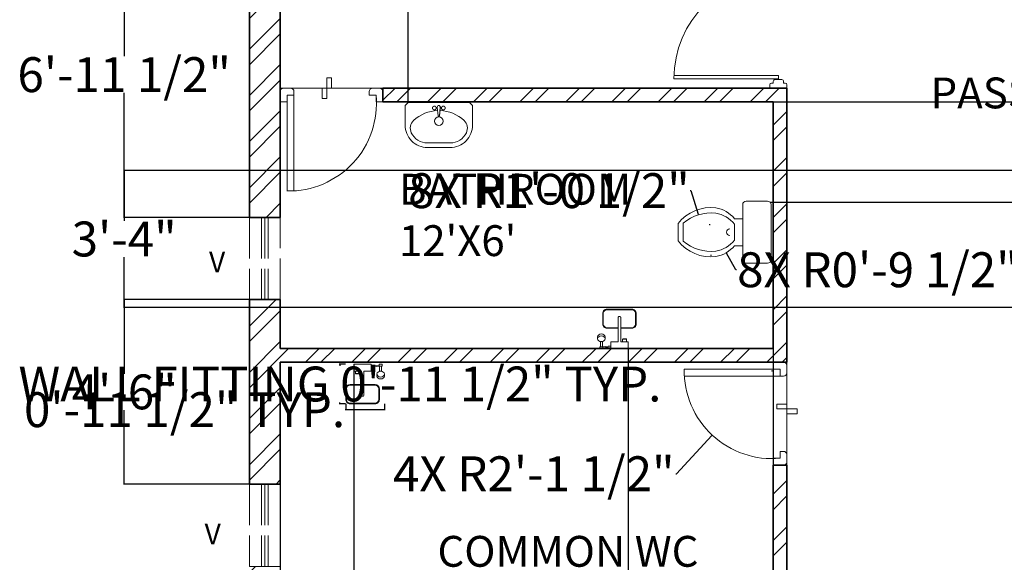
# Model space of a CAD drawing. Units: inches. Extents: x 1583 to 2239, y 1430 to 2174.
# Tile 3 of 5: x 1583 to 1871, y 1743 to 1902. Entities that reach past the tile are written whole.
import ezdxf

# ---------------------------------------------------------------- set-up
doc = ezdxf.new("R2010")
doc.units = ezdxf.units.IN
doc.linetypes.add('ACAD_ISO02W100', pattern=[15, 12, -3])
for name, color, linetype, lineweight in [('00 FURNITURE', 15, 'Continuous', 15), ('A-ANNO-DIMS', 2, 'Continuous', 18), ('A-ANNO-TEXT', 7, 'Continuous', 18), ('A-AREA-IDEN', 7, 'Continuous', 25), ('A-DOOR', 3, 'Continuous', 18), ('A-FLOR-FIXT', 9, 'Continuous', 18), ('A-GLAZ-VENT', 6, 'ACAD_ISO02W100', 13), ('A-WALL-PATT', 252, 'Continuous', 13), ('A_FUR 1', 5, 'Continuous', 5), ('WALL', 7, 'Continuous', 35)]:
    doc.layers.add(name, color=color, linetype=linetype, lineweight=lineweight)
doc.styles.get("Standard").update_dxf_attribs({"font": 'arial.ttf'})
doc.dimstyles.get("Standard").update_dxf_attribs({"dimtxt": 10.18, "dimasz": 0.18, "dimexe": 0.18, "dimexo": 0.0625, "dimgap": 0.09, "dimtad": 0, "dimtih": 1, "dimtoh": 1, "dimdec": 0, "dimzin": 0, "dimdsep": 46, "dimlunit": 3, "dimtxsty": 'Standard', "dimcen": 0.09, "dimadec": 0, "dimazin": 0, "dimtfac": 1, "dimtdec": 0, "dimtofl": 0, "dimtmove": 0, "dimatfit": 3, "dimfxl": 1, "dimtolj": 1, "dimtzin": 0, "dimarcsym": 0})

# ---------------------------------------------------------------- blocks, each defined once
blk = doc.blocks.new('DDD')
at = {"layer": '00 FURNITURE'}
for p, q in [((-12579.77, -15859.53), (-12579.77, -15829.05)), ((-12578.77, -15859.53), (-12578.77, -15829.03)), ((-12612.02, -15857.03), (-12612.02, -15862.03)), ((-12611.02, -15857.03), (-12612.02, -15857.03)), ((-12610.52, -15858.03), (-12610.52, -15857.53)), ((-12577.52, -15858.03), (-12577.52, -15857.53)), ((-12577.02, -15857.03), (-12576.02, -15857.03)), ((-12576.02, -15857.03), (-12576.02, -15862.03)), ((-12610.52, -15861.53), (-12610.52, -15861.03)), ((-12578.77, -15859.53), (-12579.77, -15859.53)), ((-12577.52, -15861.53), (-12577.52, -15861.03)), ((-12612.02, -15862.03), (-12611.02, -15862.03)), ((-12576.02, -15862.03), (-12577.02, -15862.03))]:
    blk.add_line(p, q, dxfattribs=at)
for points in [[(-12610.52, -15861.03), (-12610.02, -15861.03, 0.414214), (-12609.52, -15860.53), (-12609.52, -15858.53, 0.414214), (-12610.02, -15858.03), (-12610.52, -15858.03)], [(-12577.52, -15861.03), (-12578.02, -15861.03, -0.414214), (-12578.52, -15860.53), (-12578.52, -15858.53, -0.414214), (-12578.02, -15858.03), (-12577.52, -15858.03)]]:
    blk.add_lwpolyline(points, format="xyb", dxfattribs=at)
for centre, radius, start, end in [((-12578.77, -15859.53), 30.5, 90, 180), ((-12611.02, -15857.53), 0.5, 0, 90), ((-12577.02, -15857.53), 0.5, 90, 180), ((-12611.02, -15861.53), 0.5, 270, 0), ((-12577.02, -15861.53), 0.5, 180, 270)]:
    blk.add_arc(centre, radius, start, end, dxfattribs=at)
blk = doc.blocks.new('ESTSET')
at = {"layer": 'A_FUR 1'}
for p, q in [((-10.44, 4.1), (-10.44, 32.1)), ((-8.44, 4.1), (-8.44, 32.1)), ((-36.44, 6.1), (-36.44, 3.1)), ((-34.44, 6.1), (-36.44, 6.1)), ((-34.44, 4.1), (-34.44, 6.1)), ((-34.44, 4.1), (-34.44, 6.1)), ((-8.44, 4.1), (-8.44, 6.1)), ((-8.44, 6.1), (-6.44, 6.1)), ((-8.44, 4.1), (-8.44, 6.1)), ((-6.44, 6.1), (-6.44, 3.1)), ((-32.44, 4.1), (-34.44, 4.1)), ((-32.44, 4.1), (-34.44, 4.1)), ((-32.44, 3.1), (-32.44, 4.1)), ((-10.44, 3.1), (-10.44, 4.1)), ((-10.44, 4.1), (-8.44, 4.1)), ((-10.44, 4.1), (-8.44, 4.1)), ((-6.44, 2.1), (-36.44, 2.1)), ((-35.44, 2.1), (-33.44, 2.1)), ((-7.44, 2.1), (-9.44, 2.1))]:
    blk.add_line(p, q, dxfattribs=at)
for points in [[(-21.44, 2.1), (-18.67, 2.1), (-18.67, 5.1), (-20.06, 5.1)], [(-20.06, 5.1), (-20.06, -0.91)], [(-21.44, 2.1), (-21.44, -0.91), (-20.06, -0.91)]]:
    blk.add_lwpolyline(points, dxfattribs=at)
for centre, radius, start, end in [((-8.91, 6.46), 25.64, 88.9606, 185.2816), ((-35.44, 3.1), 1, 180, 270), ((-33.44, 3.1), 1, 270, 0), ((-9.44, 3.1), 1, 180, 270), ((-7.44, 3.1), 1, 270, 0)]:
    blk.add_arc(centre, radius, start, end, dxfattribs=at)
blk = doc.blocks.new('A$C2AC94788')
for p, q in [((0, 0.505), (0, 0.665)), ((0.025, 0.69), (0.435, 0.69)), ((0.46, 0.665), (0.46, 0.505)), ((0.435, 0.48), (0.025, 0.48)), ((0.13, 0.48), (0.13, 0.42)), ((0.33, 0.42), (0.33, 0.48)), ((0.17, 0.42), (0.29, 0.42)), ((0.1641, 0.0392), (0.2959, 0.0392)), ((0.2291, 0.0392), (0.23, 0.0392)), ((0.2309, 0.0392), (0.23, 0.0392)), ((0.165, 0), (0.295, 0))]:
    blk.add_line(p, q)
for centre, radius, start, end in [((0.025, 0.665), 0.025, 90, 180), ((0.435, 0.665), 0.025, 0, 90), ((0.025, 0.505), 0.025, 180, 270), ((0.435, 0.505), 0.025, 270, 0), ((0.2874, 0.2356), 0.2425, 130.48854, 169.44501), ((0.3274, 0.2356), 0.2425, 130.48854, 169.44501), ((0.23, 0.385), 0.025, 180, 0), ((0.1326, 0.2356), 0.2425, 10.55499, 49.51146), ((0.1726, 0.2356), 0.2425, 10.55499, 49.51146), ((0.3601, 0.2448), 0.313, 173.53688, 231.44828), ((0.4001, 0.2448), 0.313, 173.53688, 221.06038), ((0.0999, 0.2448), 0.313, 308.55172, 6.46312), ((0.0599, 0.2448), 0.313, 318.93962, 6.46312)]:
    blk.add_arc(centre, radius, start, end)
blk = doc.blocks.new('A$C7A0926BE')
for p, q in [((-6.55, 0), (-5.57, 0)), ((-6.55, -0.65), (-6.55, 0)), ((-5.57, 0), (-5.57, -0.65)), ((-2.89, 0), (-2.89, -2.29)), ((2.89, 0), (-2.89, 0)), ((2.89, -2.29), (2.89, 0)), ((-7.32, -3.29), (-7.32, -3.94)), ((-5.57, -0.65), (-6.55, -0.65)), ((-6.34, -0.65), (-5.74, -0.65)), ((-6.34, -2.33), (-6.34, -0.65)), ((-5.74, -2.33), (-6.34, -2.33)), ((-5.74, -0.65), (-5.74, -2.33)), ((-5.57, -0.28), (-2.89, -0.56)), ((-5.57, -0.65), (-2.89, -0.94)), ((-4.84, -3.94), (-4.85, -3.29)), ((-2.89, -2.29), (-0.45, -2.29)), ((0.39, -2.29), (2.89, -2.29)), ((1.04, -2.29), (1.04, -3.12)), ((2.37, -2.29), (1.04, -2.29)), ((1.04, -3.12), (2.37, -3.12)), ((1.13, -3.12), (1.13, -3.23)), ((2.3, -3.12), (1.13, -3.12)), ((1.13, -3.23), (2.3, -3.23)), ((2.3, -3.23), (2.3, -3.12)), ((2.37, -3.12), (2.37, -2.29))]:
    blk.add_line(p, q)
at = {"ltscale": 100}
for p, q in [((-0.45, -10.48), (-0.45, -2.29)), ((0.39, -10.48), (0.39, -2.29)), ((0.18, -10.69), (-0.24, -10.69))]:
    blk.add_line(p, q, dxfattribs=at)
for points in [[(-0.45, -6.79), (-4.23, -6.79, 0.414214), (-5.63, -8.19), (-5.63, -11.8, 0.414214), (-4.23, -13.2), (4.17, -13.2, 0.414214), (5.57, -11.8), (5.57, -8.19, 0.414214), (4.17, -6.79), (0.39, -6.79)], [(-0.45, -7), (-4.23, -7, 0.414214), (-5.42, -8.19), (-5.42, -11.8, 0.414214), (-4.23, -12.99), (4.17, -12.99, 0.414214), (5.36, -11.8), (5.36, -8.19, 0.414214), (4.17, -7), (0.39, -7)]]:
    blk.add_lwpolyline(points, format="xyb", dxfattribs=at)
for centre, start, end in [((-0.24, -10.48), 180, 270), ((0.18, -10.48), 270, 0)]:
    blk.add_arc(centre, 0.21, start, end, dxfattribs=at)
at = {"extrusion": (0, 0, -1)}
blk.add_ellipse((-6.08, -3.29), major_axis=(-1.24, 0), ratio=0.790849, dxfattribs=at)
blk.add_ellipse((-6.08, -3.94), major_axis=(-1.24, 0), ratio=0.790849, start_param=3.141593, end_param=6.283185, dxfattribs=at)
blk = doc.blocks.new('s_46')
at = {"ltscale": 600}
h = blk.add_hatch(color=256, dxfattribs=at)
edge = h.paths.add_edge_path()
edge.add_line((13.5, 62), (14.2, 54.1))
edge.add_ellipse((4.2, 52.3), major_axis=(-10.1, 0), ratio=1, start_angle=540, end_angle=550.17546, ccw=False)
edge.add_arc((4.2, 52.3), 10.1, 270, 360, ccw=False)
edge.add_line((4.2, 42.2), (4.2, 41.3))
edge.add_line((4.2, 41.3), (11.9, 41.3))
edge.add_arc((4.2, 52.3), 13.4, 664.69813, 766.48477)
h.paths.add_polyline_path([(4.2, 41.3), (-3.4, 41.3, 0.152567), (4.2, 38.9)])
h.paths.add_polyline_path([(11.9, 41.3), (4.2, 41.3), (4.2, 38.9, 0.152567)])
h.paths.add_polyline_path([(-5.7, 54.1), (-5, 62, 0.475833), (-3.4, 41.3), (4.2, 41.3), (4.2, 42.2, -0.46724)])
for p, q in [((-5.9, 52.3), (-0.7, 110.5)), ((-5.9, 52.3), (-0.7, 110.5)), ((9.1, 110.5), (14.2, 54.1)), ((14.3, 52.3), (9.1, 110.5)), ((14.2, 54.1), (14.3, 52.3))]:
    blk.add_line(p, q, dxfattribs=at)
blk.add_lwpolyline([(-220.8, 171.3, -0.414214), (-70.8, 321.3), (79.2, 321.3, -0.414214), (229.2, 171.3), (229.2, 41.3), (209.2, 21.3), (-200.8, 21.3), (-220.8, 41.3)], format="xyb", close=True, dxfattribs=at)
blk.add_lwpolyline([(12.3, 75.4, 0.181638), (172.2, 141.5, 0.326351), (187.7, 222.7, 0.289814), (79.2, 291.3), (-70.8, 291.3, 0.289814), (-179.2, 222.7, 0.326351), (-163.8, 141.5, 0.181638), (-3.8, 75.4)], format="xyb", dxfattribs=at)
for points in [[(-16.8, 67.4), (-17, 67.5), (-17.2, 67.6), (-17.4, 67.6), (-17.6, 67.7), (-17.8, 67.8), (-18, 67.9), (-18.1, 68.1), (-18.2, 68.2), (-18.3, 68.4), (-18.4, 68.6), (-18.5, 68.8), (-18.7, 68.9), (-18.8, 69.1), (-18.9, 69.2), (-19.1, 69.3), (-19.3, 69.3), (-19.5, 69.3), (-19.7, 69.4), (-19.9, 69.4), (-20.1, 69.4), (-20.3, 69.4), (-20.5, 69.5), (-20.7, 69.6), (-20.8, 69.7), (-21, 69.9), (-21.1, 70), (-21.3, 70.2), (-21.4, 70.3), (-21.5, 70.4), (-21.7, 70.5), (-21.9, 70.5), (-22.1, 70.5), (-22.3, 70.5), (-22.5, 70.5), (-22.7, 70.4), (-22.9, 70.4), (-23.1, 70.4), (-23.3, 70.4), (-23.5, 70.5), (-23.7, 70.6), (-23.9, 70.7), (-24, 70.8), (-24.2, 70.9), (-24.4, 71), (-24.6, 71.1), (-24.7, 71.1), (-24.9, 71.1), (-25.1, 71), (-25.3, 71), (-25.5, 70.9), (-25.7, 70.8), (-25.9, 70.7), (-26.1, 70.6), (-26.3, 70.6), (-26.5, 70.6), (-26.7, 70.6), (-26.9, 70.7), (-27.1, 70.8), (-27.3, 70.8), (-27.5, 70.9), (-27.7, 70.9), (-27.8, 70.9), (-28, 70.8), (-28.2, 70.8), (-28.3, 70.6), (-28.5, 70.5), (-28.7, 70.4), (-28.9, 70.3), (-29.1, 70.2), (-29.3, 70.1), (-29.6, 70.1), (-29.9, 70.1), (-30.2, 70.1), (-30.5, 70), (-30.8, 69.8), (-31.1, 69.5), (-31.4, 69), (-31.6, 68.4), (-32.3, 68.5), (-32.8, 68.4), (-33.2, 68.3), (-33.5, 68.1), (-33.7, 67.8), (-33.9, 67.6), (-34, 67.3), (-34.1, 67.1), (-34.3, 66.9), (-34.5, 66.7), (-34.7, 66.6), (-34.9, 66.5), (-35.1, 66.4), (-35.2, 66.3), (-35.4, 66.2), (-35.5, 66), (-35.6, 65.9), (-35.6, 65.7), (-35.7, 65.5), (-35.7, 65.3), (-35.7, 65.1), (-35.8, 64.9), (-35.8, 64.7), (-35.9, 64.5), (-36, 64.3), (-36.2, 64.2), (-36.3, 64), (-36.5, 63.9), (-36.6, 63.8), (-36.8, 63.6), (-36.9, 63.5), (-37, 63.3), (-37, 63.1), (-37, 63), (-37, 62.8), (-37, 62.6), (-37, 62.3), (-37, 62.1), (-37, 61.9), (-37, 61.7), (-37.1, 61.5), (-37.2, 61.4), (-37.3, 61.2), (-37.4, 61), (-37.5, 60.8), (-37.6, 60.7), (-37.7, 60.5), (-37.8, 60.3), (-37.8, 60.1), (-37.7, 60), (-37.7, 59.8), (-37.6, 59.6), (-37.5, 59.4), (-37.4, 59.2), (-37.4, 59), (-37.4, 58.8), (-37.4, 58.6), (-37.4, 58.4), (-37.5, 58.2), (-37.6, 58), (-37.7, 57.8), (-37.7, 57.6), (-37.8, 57.4), (-37.8, 57.2), (-37.7, 57.1), (-37.6, 56.9), (-37.5, 56.7), (-37.4, 56.6), (-37.3, 56.4), (-37.2, 56.2), (-37.1, 56), (-37, 55.8), (-37, 55.6), (-37, 55.4), (-37, 55.2), (-37, 55), (-37, 54.8), (-37, 54.6), (-37, 54.4), (-37, 54.2), (-36.9, 54.1), (-36.8, 53.9), (-36.6, 53.8), (-36.5, 53.7), (-36.3, 53.5), (-36.2, 53.4), (-36, 53.2), (-35.9, 53.1), (-35.8, 52.9), (-35.8, 52.7), (-35.7, 52.5), (-35.7, 52.3), (-35.7, 52.1), (-35.6, 51.9), (-35.6, 51.7), (-35.5, 51.5), (-35.4, 51.4), (-35.2, 51.3), (-35.1, 51.2), (-34.9, 51.1), (-34.7, 51), (-34.5, 50.9), (-34.3, 50.8), (-34.2, 50.7), (-34, 50.5), (-33.9, 50.3), (-33.8, 50.1), (-33.8, 49.9), (-33.7, 49.8), (-33.6, 49.6), (-33.5, 49.4), (-33.4, 49.3), (-33.2, 49.2), (-33.1, 49.1), (-32.9, 49.1), (-32.7, 49), (-32.5, 49), (-32.2, 48.9), (-32.1, 48.9), (-31.9, 48.8), (-31.7, 48.7), (-31.6, 48.5), (-31.4, 48.3), (-31.3, 48.2), (-31.2, 48), (-31.1, 47.9), (-30.9, 47.7), (-30.8, 47.6), (-30.6, 47.6), (-30.4, 47.5), (-30.2, 47.5), (-30, 47.6), (-29.8, 47.6), (-29.6, 47.6), (-29.4, 47.6), (-29.2, 47.5), (-29, 47.4), (-28.8, 47.3), (-28.7, 47.2), (-28.5, 47.1), (-28.3, 46.9), (-28.2, 46.8), (-28, 46.7), (-27.8, 46.7), (-27.7, 46.7), (-27.5, 46.7), (-27.3, 46.7), (-27.1, 46.8), (-26.9, 46.9), (-26.7, 46.9), (-26.5, 47), (-26.3, 47), (-26.1, 46.9), (-25.9, 46.9), (-25.7, 46.8), (-25.5, 46.7), (-25.3, 46.6), (-25.1, 46.5), (-24.9, 46.5), (-24.7, 46.5), (-24.6, 46.5), (-24.4, 46.6), (-24.2, 46.7), (-24, 46.8), (-23.9, 46.9), (-23.7, 47), (-23.5, 47.1), (-23.3, 47.1), (-23.1, 47.2), (-22.9, 47.2), (-22.7, 47.1), (-22.5, 47.1), (-22.3, 47), (-22.1, 47), (-21.9, 47), (-21.7, 47.1), (-21.5, 47.1), (-21.4, 47.2), (-21.3, 47.4), (-21.1, 47.5), (-21, 47.7), (-20.8, 47.8), (-20.7, 48), (-20.5, 48.1), (-20.3, 48.1), (-20.1, 48.2), (-19.9, 48.2), (-19.7, 48.2), (-19.5, 48.2), (-19.3, 48.2), (-19.1, 48.3), (-18.9, 48.4), (-18.8, 48.5), (-18.7, 48.6), (-18.5, 48.8), (-18.4, 49), (-18.3, 49.2), (-18.2, 49.3), (-18.1, 49.5), (-18, 49.7), (-17.8, 49.8), (-17.6, 49.9), (-17.4, 49.9), (-17.2, 50), (-17, 50.1), (-16.8, 50.1), (-16.7, 50.2), (-16.5, 50.3), (-16.4, 50.5), (-16.3, 50.7), (-16.3, 50.8), (-16.2, 51), (-16.2, 51.3), (-16.1, 51.5), (-16, 51.6), (-15.9, 51.8), (-15.8, 52), (-15.6, 52.1), (-15.5, 52.2), (-15.3, 52.3), (-15.1, 52.4), (-15, 52.6), (-14.8, 52.7), (-14.7, 52.8), (-14.7, 53), (-14.6, 53.2), (-14.6, 53.4), (-14.6, 53.6), (-14.6, 53.8), (-14.6, 54), (-14.6, 54.2), (-14.5, 54.4), (-14.4, 54.6), (-14.3, 54.8), (-14.2, 54.9), (-14, 55.1), (-13.9, 55.2), (-13.7, 55.4), (-13.6, 55.5), (-13.6, 55.7), (-13.6, 55.9), (-13.6, 56.1), (-13.6, 56.3), (-13.7, 56.5), (-13.7, 56.7), (-13.8, 56.9), (-13.8, 57.1), (-13.8, 57.3), (-13.7, 57.5), (-13.7, 57.7), (-13.6, 57.9), (-13.5, 58.1), (-13.4, 58.2), (-13.3, 58.4), (-13.2, 58.6), (-13.2, 58.8), (-13.2, 59), (-13.3, 59.1), (-13.4, 59.3), (-13.5, 59.5), (-13.6, 59.7), (-13.7, 59.9), (-13.7, 60.1), (-13.8, 60.3), (-13.8, 60.5), (-13.8, 60.7), (-13.7, 60.9), (-13.7, 61.1), (-13.6, 61.3), (-13.6, 61.5), (-13.6, 61.7), (-13.6, 61.9), (-13.6, 62), (-13.7, 62.2), (-13.9, 62.3), (-14, 62.5), (-14.2, 62.6), (-14.3, 62.8), (-14.4, 63), (-14.5, 63.1), (-14.6, 63.3), (-14.6, 63.5), (-14.6, 63.8), (-14.6, 64), (-14.6, 64.2), (-14.6, 64.4), (-14.7, 64.6), (-14.7, 64.7), (-14.8, 64.9), (-15, 65), (-15.1, 65.1), (-15.3, 65.2), (-15.5, 65.3), (-15.6, 65.5), (-15.8, 65.6), (-15.9, 65.7), (-16, 65.9), (-16.1, 66.1), (-16.2, 66.3), (-16.2, 66.5), (-16.3, 66.7), (-16.3, 66.9), (-16.4, 67.1), (-16.5, 67.2), (-16.7, 67.3)], [(22.1, 61.1), (22, 61.3), (22, 61.5), (22, 61.7), (22, 61.9), (22.1, 62), (22.2, 62.2), (22.3, 62.3), (22.4, 62.5), (22.6, 62.6), (22.7, 62.8), (22.8, 63), (22.9, 63.1), (23, 63.3), (23, 63.5), (23, 63.8), (23, 64), (23, 64.2), (23, 64.4), (23.1, 64.6), (23.1, 64.7), (23.2, 64.9), (23.4, 65), (23.5, 65.1), (23.7, 65.2), (23.9, 65.3), (24.1, 65.5), (24.2, 65.6), (24.4, 65.7), (24.5, 65.9), (24.5, 66.1), (24.6, 66.3), (24.7, 66.5), (24.7, 66.7), (24.8, 66.9), (24.9, 67.1), (25, 67.2), (25.1, 67.3), (25.3, 67.4), (25.4, 67.5), (25.6, 67.6), (25.8, 67.6), (26, 67.7), (26.2, 67.8), (26.4, 67.9), (26.5, 68.1), (26.7, 68.2), (26.8, 68.4), (26.9, 68.6), (27, 68.8), (27.1, 68.9), (27.2, 69.1), (27.3, 69.2), (27.5, 69.3), (27.7, 69.3), (27.9, 69.3), (28.1, 69.4), (28.3, 69.4), (28.5, 69.4), (28.7, 69.4), (28.9, 69.5), (29.1, 69.6), (29.2, 69.7), (29.4, 69.9), (29.5, 70), (29.7, 70.2), (29.8, 70.3), (30, 70.4), (30.1, 70.5), (30.3, 70.5), (30.5, 70.5), (30.7, 70.5), (30.9, 70.5), (31.1, 70.4), (31.3, 70.4), (31.5, 70.4), (31.7, 70.4), (31.9, 70.5), (32.1, 70.6), (32.3, 70.7), (32.5, 70.8), (32.6, 70.9), (32.8, 71), (33, 71.1), (33.2, 71.1), (33.4, 71.1), (33.5, 71), (33.7, 71), (33.9, 70.9), (34.1, 70.8), (34.3, 70.7), (34.5, 70.6), (34.7, 70.6), (34.9, 70.6), (35.1, 70.6), (35.3, 70.7), (35.5, 70.8), (35.7, 70.8), (35.9, 70.9), (36.1, 70.9), (36.3, 70.9), (36.4, 70.8), (36.6, 70.8), (36.8, 70.6), (36.9, 70.5), (37.1, 70.4), (37.3, 70.3), (37.5, 70.2), (37.8, 70.1), (38, 70.1), (38.3, 70.1), (38.6, 70.1), (38.9, 70), (39.2, 69.8), (39.5, 69.5), (39.8, 69), (40.1, 68.4), (40.7, 68.5), (41.3, 68.4), (41.7, 68.3), (42, 68.1), (42.2, 67.8), (42.3, 67.6), (42.4, 67.3), (42.6, 67.1), (42.7, 66.9), (42.9, 66.7), (43.1, 66.6), (43.3, 66.5), (43.5, 66.4), (43.6, 66.3), (43.8, 66.2), (43.9, 66), (44, 65.9), (44.1, 65.7), (44.1, 65.5), (44.1, 65.3), (44.2, 65.1), (44.2, 64.9), (44.2, 64.7), (44.3, 64.5), (44.4, 64.3), (44.6, 64.2), (44.7, 64), (44.9, 63.9), (45.1, 63.8), (45.2, 63.6), (45.3, 63.5), (45.4, 63.3), (45.5, 63.1), (45.5, 63), (45.5, 62.8), (45.4, 62.6), (45.4, 62.3), (45.4, 62.1), (45.4, 61.9), (45.4, 61.7), (45.5, 61.5), (45.6, 61.4), (45.7, 61.2), (45.8, 61), (46, 60.8), (46.1, 60.7), (46.1, 60.5), (46.2, 60.3), (46.2, 60.1), (46.1, 60), (46.1, 59.8), (46, 59.6), (45.9, 59.4), (45.9, 59.2), (45.8, 59), (45.8, 58.8), (45.8, 58.6), (45.9, 58.4), (45.9, 58.2), (46, 58), (46.1, 57.8), (46.1, 57.6), (46.2, 57.4), (46.2, 57.2), (46.1, 57.1), (46.1, 56.9), (46, 56.7), (45.8, 56.6), (45.7, 56.4), (45.6, 56.2), (45.5, 56), (45.4, 55.8), (45.4, 55.6), (45.4, 55.4), (45.4, 55.2), (45.4, 55), (45.5, 54.8), (45.5, 54.6), (45.5, 54.4), (45.4, 54.2), (45.3, 54.1), (45.2, 53.9), (45.1, 53.8), (44.9, 53.7), (44.7, 53.5), (44.6, 53.4), (44.4, 53.2), (44.3, 53.1), (44.2, 52.9), (44.2, 52.7), (44.2, 52.5), (44.1, 52.3), (44.1, 52.1), (44.1, 51.9), (44, 51.7), (43.9, 51.5), (43.8, 51.4), (43.6, 51.3), (43.5, 51.2), (43.3, 51.1), (43.1, 51), (42.9, 50.9), (42.7, 50.8), (42.6, 50.7), (42.5, 50.5), (42.4, 50.3), (42.3, 50.1), (42.2, 49.9), (42.1, 49.8), (42, 49.6), (41.9, 49.4), (41.8, 49.3), (41.7, 49.2), (41.5, 49.1), (41.3, 49.1), (41.1, 49), (40.9, 49), (40.7, 48.9), (40.5, 48.9), (40.3, 48.8), (40.1, 48.7), (40, 48.5), (39.9, 48.3), (39.7, 48.2), (39.6, 48), (39.5, 47.9), (39.4, 47.7), (39.2, 47.6), (39, 47.6), (38.8, 47.5), (38.6, 47.5), (38.4, 47.6), (38.2, 47.6), (38, 47.6), (37.8, 47.6), (37.6, 47.5), (37.4, 47.4), (37.2, 47.3), (37.1, 47.2), (36.9, 47.1), (36.8, 46.9), (36.6, 46.8), (36.4, 46.7), (36.3, 46.7), (36.1, 46.7), (35.9, 46.7), (35.7, 46.7), (35.5, 46.8), (35.3, 46.9), (35.1, 46.9), (34.9, 47), (34.7, 47), (34.5, 46.9), (34.3, 46.9), (34.1, 46.8), (33.9, 46.7), (33.7, 46.6), (33.5, 46.5), (33.4, 46.5), (33.2, 46.5), (33, 46.5), (32.8, 46.6), (32.6, 46.7), (32.5, 46.8), (32.3, 46.9), (32.1, 47), (31.9, 47.1), (31.7, 47.1), (31.5, 47.2), (31.3, 47.2), (31.1, 47.1), (30.9, 47.1), (30.7, 47), (30.5, 47), (30.3, 47), (30.1, 47.1), (30, 47.1), (29.8, 47.2), (29.7, 47.4), (29.5, 47.5), (29.4, 47.7), (29.2, 47.8), (29.1, 48), (28.9, 48.1), (28.7, 48.1), (28.5, 48.2), (28.3, 48.2), (28.1, 48.2), (27.9, 48.2), (27.7, 48.2), (27.5, 48.3), (27.3, 48.4), (27.2, 48.5), (27.1, 48.6), (27, 48.8), (26.9, 49), (26.8, 49.2), (26.7, 49.3), (26.5, 49.5), (26.4, 49.7), (26.2, 49.8), (26, 49.9), (25.8, 49.9), (25.6, 50), (25.4, 50.1), (25.3, 50.1), (25.1, 50.2), (25, 50.3), (24.9, 50.5), (24.8, 50.7), (24.7, 50.8), (24.7, 51), (24.6, 51.3), (24.5, 51.5), (24.5, 51.6), (24.4, 51.8), (24.2, 52), (24.1, 52.1), (23.9, 52.2), (23.7, 52.3), (23.5, 52.4), (23.4, 52.6), (23.2, 52.7), (23.1, 52.8), (23.1, 53), (23, 53.2), (23, 53.4), (23, 53.6), (23, 53.8), (23, 54), (23, 54.2), (22.9, 54.4), (22.8, 54.6), (22.7, 54.8), (22.6, 54.9), (22.4, 55.1), (22.3, 55.2), (22.2, 55.4), (22.1, 55.5), (22, 55.7), (22, 55.9), (22, 56.1), (22, 56.3), (22.1, 56.5), (22.1, 56.7), (22.2, 56.9), (22.2, 57.1), (22.2, 57.3), (22.2, 57.5), (22.1, 57.7), (22, 57.9), (21.9, 58.1), (21.8, 58.2), (21.7, 58.4), (21.6, 58.6), (21.6, 58.8), (21.6, 59), (21.7, 59.1), (21.8, 59.3), (21.9, 59.5), (22, 59.7), (22.1, 59.9), (22.2, 60.1), (22.2, 60.3), (22.2, 60.5), (22.2, 60.7), (22.1, 60.9)]]:
    blk.add_lwpolyline(points, close=True, dxfattribs=at)
blk.add_circle((4.2, 146.3), 28, dxfattribs=at)
for centre, radius, start, end in [((4.2, 108.2), 5.42, 24.6783, 155.3217), ((4.2, 52.3), 10.1, 169.82454, 0)]:
    blk.add_arc(centre, radius, start, end, dxfattribs=at)
for centre, major_axis, ratio, start_param, end_param in [((4.2, 110.5), (-4.93, 0), 0.641024, 3.141593, 6.283185), ((4.2, 52.3), (-10.1, 0), 1, 6.10559, 9.602373)]:
    blk.add_ellipse(centre, major_axis=major_axis, ratio=ratio, start_param=start_param, end_param=end_param, dxfattribs=at)
blk = doc.blocks.new('VENT-GRILLE-24IN')
for p, q in [((24, 2), (0, 2)), ((24, 1), (0, 1)), ((24, 0), (0, 0))]:
    blk.add_line(p, q)
blk = doc.blocks.new('*D25')
at = {"layer": 'A-ANNO-DIMS', "color": 0, "lineweight": -2, "transparency": 16777216}
for p, q in [((1678.62, 1801.07), (1676.78, 1801.07)), ((1676.96, 1800.89), (1676.96, 1800.66)), ((1678.62, 1789.55), (1676.78, 1789.55)), ((1676.96, 1789.73), (1676.96, 1789.96))]:
    blk.add_line(p, q, dxfattribs=at)
at = {"layer": 'A-ANNO-DIMS', "color": 0, "transparency": 16777216}
for points in [[(1676.93, 1800.89), (1676.99, 1800.89), (1676.96, 1801.07)], [(1676.93, 1789.73), (1676.99, 1789.73), (1676.96, 1789.55)]]:
    blk.add_solid(points, dxfattribs=at)
at = {"layer": 'Defpoints', "color": 0, "transparency": 16777216}
for p in [(1676.96, 1801.07), (1678.69, 1801.07), (1678.69, 1789.55)]:
    blk.add_point(p, dxfattribs=at)
at = {"layer": 'A-ANNO-DIMS', "color": 0, "transparency": 16777216, "insert": (1676.96, 1795.31), "char_height": 10.18, "attachment_point": 5}
blk.add_mtext('\\A1;WALL FITTING 0\'-11 1/2" TYP.', dxfattribs=at)
blk = doc.blocks.new('*D26')
at = {"layer": 'A-ANNO-DIMS', "color": 0, "lineweight": -2, "transparency": 16777216}
for p, q in [((1678.69, 1789.48), (1678.69, 1787.64)), ((1689.95, 1789.48), (1689.95, 1787.64)), ((1678.69, 1787.82), (1678.51, 1787.82)), ((1689.77, 1787.82), (1678.87, 1787.82))]:
    blk.add_line(p, q, dxfattribs=at)
at = {"layer": 'A-ANNO-DIMS', "color": 0, "transparency": 16777216}
for points in [[(1678.87, 1787.85), (1678.87, 1787.79), (1678.69, 1787.82)], [(1689.77, 1787.85), (1689.77, 1787.79), (1689.95, 1787.82)]]:
    blk.add_solid(points, dxfattribs=at)
at = {"layer": 'Defpoints', "color": 0, "transparency": 16777216}
for p in [(1678.69, 1789.55), (1689.95, 1789.55), (1678.69, 1787.82)]:
    blk.add_point(p, dxfattribs=at)
at = {"layer": 'A-ANNO-DIMS', "color": 0, "transparency": 16777216, "insert": (1631.57, 1787.82), "char_height": 10.18, "attachment_point": 5}
blk.add_mtext('\\A1;0\'-11 1/2" TYP.', dxfattribs=at)
blk = doc.blocks.new('*D38')
at = {"layer": 'A-ANNO-DIMS', "color": 0, "lineweight": -2, "transparency": 16777216}
for p, q in [((1650.47, 1819.95), (1613.75, 1819.95)), ((1613.93, 1819.77), (1613.93, 1798.3)), ((1613.93, 1766.26), (1613.93, 1787.72)), ((1650.47, 1766.08), (1613.75, 1766.08))]:
    blk.add_line(p, q, dxfattribs=at)
at = {"layer": 'A-ANNO-DIMS', "color": 0, "transparency": 16777216}
for points in [[(1613.9, 1819.77), (1613.96, 1819.77), (1613.93, 1819.95)], [(1613.9, 1766.26), (1613.96, 1766.26), (1613.93, 1766.08)]]:
    blk.add_solid(points, dxfattribs=at)
at = {"layer": 'Defpoints', "color": 0, "transparency": 16777216}
for p in [(1613.93, 1819.95), (1650.53, 1819.95), (1650.53, 1766.08)]:
    blk.add_point(p, dxfattribs=at)
at = {"layer": 'A-ANNO-DIMS', "color": 0, "transparency": 16777216, "insert": (1613.93, 1793.01), "char_height": 10.18, "attachment_point": 5}
blk.add_mtext('\\A1;4\'-6"', dxfattribs=at)
blk = doc.blocks.new('*D39')
at = {"layer": 'A-ANNO-DIMS', "color": 0, "lineweight": -2, "transparency": 16777216}
for p, q in [((1650.47, 1927.26), (1613.75, 1927.26)), ((1613.93, 1927.08), (1613.93, 1890.96)), ((1613.93, 1844.13), (1613.93, 1880.25)), ((1650.47, 1843.95), (1613.75, 1843.95))]:
    blk.add_line(p, q, dxfattribs=at)
at = {"layer": 'A-ANNO-DIMS', "color": 0, "transparency": 16777216}
for points in [[(1613.9, 1927.08), (1613.96, 1927.08), (1613.93, 1927.26)], [(1613.9, 1844.13), (1613.96, 1844.13), (1613.93, 1843.95)]]:
    blk.add_solid(points, dxfattribs=at)
at = {"layer": 'Defpoints', "color": 0, "transparency": 16777216}
for p in [(1613.93, 1927.26), (1650.53, 1927.26), (1650.53, 1843.95)]:
    blk.add_point(p, dxfattribs=at)
at = {"layer": 'A-ANNO-DIMS', "color": 0, "transparency": 16777216, "insert": (1613.93, 1885.6), "char_height": 10.18, "attachment_point": 5}
blk.add_mtext('\\A1;6\'-11 1/2"', dxfattribs=at)
blk = doc.blocks.new('*D44')
at = {"layer": 'A-ANNO-DIMS', "color": 0, "lineweight": -2, "transparency": 16777216}
for p, q in [((1953.47, 1857.64), (1613.75, 1857.64)), ((1613.93, 1857.46), (1613.93, 1842.93)), ((1613.93, 1817.82), (1613.93, 1832.35)), ((1953.47, 1817.64), (1613.75, 1817.64))]:
    blk.add_line(p, q, dxfattribs=at)
at = {"layer": 'A-ANNO-DIMS', "color": 0, "transparency": 16777216}
for points in [[(1613.9, 1857.46), (1613.96, 1857.46), (1613.93, 1857.64)], [(1613.9, 1817.82), (1613.96, 1817.82), (1613.93, 1817.64)]]:
    blk.add_solid(points, dxfattribs=at)
at = {"layer": 'Defpoints', "color": 0, "transparency": 16777216}
for p in [(1613.93, 1857.64), (1953.53, 1857.64), (1953.53, 1817.64)]:
    blk.add_point(p, dxfattribs=at)
at = {"layer": 'A-ANNO-DIMS', "color": 0, "transparency": 16777216, "insert": (1613.93, 1837.64), "char_height": 10.18, "attachment_point": 5}
blk.add_mtext('\\A1;3\'-4"', dxfattribs=at)
blk = doc.blocks.new('*D55')
at = {"layer": 'A-ANNO-DIMS', "color": 0, "lineweight": -2, "transparency": 16777216}
for p, q in [((1659.53, 1877.7), (1659.53, 2159.42)), ((1659.71, 2159.24), (1696.67, 2159.24)), ((1696.85, 1877.57), (1696.85, 2159.42)), ((1696.85, 2159.24), (1697.03, 2159.24))]:
    blk.add_line(p, q, dxfattribs=at)
at = {"layer": 'A-ANNO-DIMS', "color": 0, "transparency": 16777216}
for points in [[(1659.71, 2159.27), (1659.71, 2159.21), (1659.53, 2159.24)], [(1696.67, 2159.27), (1696.67, 2159.21), (1696.85, 2159.24)]]:
    blk.add_solid(points, dxfattribs=at)
at = {"layer": 'Defpoints', "color": 0, "transparency": 16777216}
for p in [(1696.85, 2159.24), (1659.53, 1877.64), (1696.85, 1877.51)]:
    blk.add_point(p, dxfattribs=at)
at = {"layer": 'A-ANNO-DIMS', "color": 0, "transparency": 16777216, "insert": (1722.51, 2159.24), "char_height": 10.18, "attachment_point": 5}
blk.add_mtext('\\A1;3\'-1 1/2"', dxfattribs=at)
blk = doc.blocks.new('*D56')
at = {"layer": 'A-ANNO-DIMS', "color": 0, "lineweight": -2, "transparency": 16777216}
for p, q in [((1803.59, 1877.64), (2167.31, 1877.64)), ((2167.13, 1877.46), (2167.13, 1868.3)), ((2167.13, 1848.57), (2167.13, 1857.73)), ((1802.65, 1848.39), (2167.31, 1848.39))]:
    blk.add_line(p, q, dxfattribs=at)
at = {"layer": 'A-ANNO-DIMS', "color": 0, "transparency": 16777216}
for points in [[(2167.1, 1877.46), (2167.16, 1877.46), (2167.13, 1877.64)], [(2167.1, 1848.57), (2167.16, 1848.57), (2167.13, 1848.39)]]:
    blk.add_solid(points, dxfattribs=at)
at = {"layer": 'Defpoints', "color": 0, "transparency": 16777216}
for p in [(1803.53, 1877.64), (1802.59, 1848.39), (2167.13, 1848.39)]:
    blk.add_point(p, dxfattribs=at)
at = {"layer": 'A-ANNO-DIMS', "color": 0, "transparency": 16777216, "insert": (2167.13, 1863.01), "char_height": 10.18, "attachment_point": 5}
blk.add_mtext('\\A1;2\'-5"', dxfattribs=at)
blk = doc.blocks.new('*D59')
at = {"layer": 'A-ANNO-DIMS', "color": 0, "lineweight": -2, "transparency": 16777216}
for p, q in [((1659.53, 1801.58), (1659.53, 1485.86)), ((1681.03, 1801.01), (1681.03, 1485.86)), ((1659.71, 1486.04), (1680.85, 1486.04)), ((1681.03, 1486.04), (1681.21, 1486.04))]:
    blk.add_line(p, q, dxfattribs=at)
at = {"layer": 'A-ANNO-DIMS', "color": 0, "transparency": 16777216}
for points in [[(1659.71, 1486.07), (1659.71, 1486.01), (1659.53, 1486.04)], [(1680.85, 1486.07), (1680.85, 1486.01), (1681.03, 1486.04)]]:
    blk.add_solid(points, dxfattribs=at)
at = {"layer": 'Defpoints', "color": 0, "transparency": 16777216}
for p in [(1659.53, 1801.64), (1681.03, 1801.07), (1681.03, 1486.04)]:
    blk.add_point(p, dxfattribs=at)
at = {"layer": 'A-ANNO-DIMS', "color": 0, "transparency": 16777216, "insert": (1706.21, 1486.04), "char_height": 10.18, "attachment_point": 5}
blk.add_mtext('\\A1;1\'-9 1/2"', dxfattribs=at)
blk = doc.blocks.new('*D60')
at = {"layer": 'A-ANNO-DIMS', "color": 0, "lineweight": -2, "transparency": 16777216}
for p, q in [((1761.15, 1805.58), (1761.15, 1485.86)), ((1803.53, 1805.58), (1803.53, 1485.86)), ((1761.33, 1486.04), (1803.35, 1486.04)), ((1803.53, 1486.04), (1803.71, 1486.04))]:
    blk.add_line(p, q, dxfattribs=at)
at = {"layer": 'A-ANNO-DIMS', "color": 0, "transparency": 16777216}
for points in [[(1761.33, 1486.07), (1761.33, 1486.01), (1761.15, 1486.04)], [(1803.35, 1486.07), (1803.35, 1486.01), (1803.53, 1486.04)]]:
    blk.add_solid(points, dxfattribs=at)
at = {"layer": 'Defpoints', "color": 0, "transparency": 16777216}
for p in [(1761.15, 1805.64), (1803.53, 1805.64), (1803.53, 1486.04)]:
    blk.add_point(p, dxfattribs=at)
at = {"layer": 'A-ANNO-DIMS', "color": 0, "transparency": 16777216, "insert": (1829.19, 1486.04), "char_height": 10.18, "attachment_point": 5}
blk.add_mtext('\\A1;3\'-6 1/2"', dxfattribs=at)
blk = doc.blocks.new('*D62')
at = {"layer": 'A-ANNO-DIMS', "color": 0, "lineweight": -2, "transparency": 16777216}
for p, q in [((1803.08, 1799.17), (1803.26, 1799.17)), ((1803.17, 1799.08), (1803.17, 1799.26)), ((1775.25, 1769.11), (1785.6, 1780.25)), ((1775.07, 1769.11), (1775.25, 1769.11))]:
    blk.add_line(p, q, dxfattribs=at)
at = {"layer": 'A-ANNO-DIMS', "color": 0, "transparency": 16777216}
blk.add_solid([(1785.58, 1780.27), (1785.62, 1780.23), (1785.72, 1780.38)], dxfattribs=at)
at = {"layer": 'Defpoints', "color": 0, "transparency": 16777216}
for p in [(1803.17, 1799.17), (1785.72, 1780.38)]:
    blk.add_point(p, dxfattribs=at)
at = {"layer": 'A-ANNO-DIMS', "color": 0, "transparency": 16777216, "insert": (1733.58, 1769.11), "char_height": 10.18, "attachment_point": 5}
blk.add_mtext('\\A1;4X R2\'-1 1/2"', dxfattribs=at)
blk = doc.blocks.new('*D64')
at = {"layer": 'A-ANNO-DIMS', "color": 0, "lineweight": -2, "transparency": 16777216}
for p, q in [((1779.3, 1851.75), (1779.48, 1851.75)), ((1779.48, 1851.75), (1781.63, 1844.86)), ((1785.26, 1832.93), (1785.44, 1832.93)), ((1785.35, 1832.84), (1785.35, 1833.02))]:
    blk.add_line(p, q, dxfattribs=at)
at = {"layer": 'A-ANNO-DIMS', "color": 0, "transparency": 16777216}
blk.add_solid([(1781.66, 1844.87), (1781.6, 1844.86), (1781.68, 1844.69)], dxfattribs=at)
at = {"layer": 'Defpoints', "color": 0, "transparency": 16777216}
for p in [(1781.68, 1844.69), (1785.35, 1832.93)]:
    blk.add_point(p, dxfattribs=at)
at = {"layer": 'A-ANNO-DIMS', "color": 0, "transparency": 16777216, "insert": (1738.01, 1851.75), "char_height": 10.18, "attachment_point": 5}
blk.add_mtext('\\A1;8X R1\'-0 1/2"', dxfattribs=at)
blk = doc.blocks.new('*D65')
at = {"layer": 'A-ANNO-DIMS', "color": 0, "lineweight": -2, "transparency": 16777216}
for p, q in [((1784.89, 1841.88), (1785.07, 1841.88)), ((1784.98, 1841.79), (1784.98, 1841.97)), ((1792.63, 1828.66), (1789.85, 1833.46)), ((1792.81, 1828.66), (1792.63, 1828.66))]:
    blk.add_line(p, q, dxfattribs=at)
at = {"layer": 'A-ANNO-DIMS', "color": 0, "transparency": 16777216}
blk.add_solid([(1789.88, 1833.48), (1789.83, 1833.45), (1789.76, 1833.62)], dxfattribs=at)
at = {"layer": 'Defpoints', "color": 0, "transparency": 16777216}
for p in [(1784.98, 1841.88), (1789.76, 1833.62)]:
    blk.add_point(p, dxfattribs=at)
at = {"layer": 'A-ANNO-DIMS', "color": 0, "transparency": 16777216, "insert": (1834.11, 1828.66), "char_height": 10.18, "attachment_point": 5}
blk.add_mtext('\\A1;8X R0\'-9 1/2"', dxfattribs=at)

msp = doc.modelspace()

# ---------------------------------------------------------------- hatches: boundary and pattern name
at = {"layer": 'A-WALL-PATT'}
h = msp.add_hatch(dxfattribs=at)
h.set_pattern_fill('ANSI32', color=256)
h.paths.add_polyline_path([(1715.9, 2122.64), (1650.53, 2122.64), (1650.53, 1975.26), (1659.53, 1975.26), (1659.53, 1975.26), (1659.53, 2013.64), (1803.53, 2013.64), (1803.53, 1917.64), (1807.53, 1917.64), (1807.53, 2013.64), (1839.53, 2013.64), (1839.53, 2017.64), (1659.53, 2017.64), (1659.53, 2113.64), (1715.9, 2113.64)])
h.paths.add_polyline_path([(1893.86, 2122.64), (1763.9, 2122.64), (1763.9, 2113.64), (1875.53, 2113.64), (1875.53, 2013.64), (1879.53, 2013.64), (1879.53, 2037.64), (1909.53, 2037.64), (1909.53, 2041.64), (1879.53, 2041.64), (1879.53, 2113.64), (1893.86, 2113.64)])
h.paths.add_polyline_path([(1999.8, 2122.64), (1917.86, 2122.64), (1917.86, 2113.64), (1939.53, 2113.64), (1939.53, 2037.64), (1939.53, 1941.64), (1943.53, 1941.64), (1943.53, 2049.64), (2091.53, 2049.64), (2091.53, 2053.64), (1943.53, 2053.64), (1943.53, 2113.64), (1999.8, 2113.64)])
h.paths.add_polyline_path([(2130.53, 2122.64), (2023.8, 2122.64), (2023.8, 2113.64), (2121.53, 2113.64), (2121.53, 2049.64), (2121.53, 2013.82), (2130.53, 2013.82), (2130.53, 2013.82)])
h.paths.add_polyline_path([(2130.53, 1965.82), (2121.53, 1965.82), (2121.53, 1905.64), (1944.53, 1905.64), (1944.53, 1905.64), (1939.53, 1905.64), (1939.53, 1901.64), (2121.53, 1901.64), (2121.53, 1879.63), (2130.53, 1879.63)])
h.paths.add_polyline_path([(2130.53, 1855.63), (2121.53, 1855.63), (2121.53, 1817.64), (1939.53, 1817.64), (1939.53, 1729.64), (1943.53, 1729.64), (1943.53, 1813.64), (2121.53, 1813.64), (2121.53, 1780.2), (2130.53, 1780.2), (2130.53, 1780.2)])
h.paths.add_polyline_path([(2130.53, 1732.2), (2121.53, 1732.2), (2121.53, 1693.64), (1944.53, 1693.64), (1944.53, 1693.64), (1939.53, 1693.64), (1900.39, 1693.64), (1900.39, 1689.64), (2121.53, 1689.64), (2121.53, 1649.31), (2130.53, 1649.31), (2130.53, 1649.31)])
h.paths.add_polyline_path([(2130.53, 1601.31), (2121.53, 1601.31), (2121.53, 1531.64), (2056.46, 1531.64), (2056.46, 1522.64), (2130.53, 1522.64)])
h.paths.add_polyline_path([(2032.46, 1531.64), (1943.39, 1531.64), (1943.39, 1526.25), (1943.39, 1526.25), (1943.39, 1522.64), (2032.46, 1522.64)])
h.paths.add_polyline_path([(1895.39, 1531.64), (1871.02, 1531.64), (1871.02, 1522.64), (1895.39, 1522.64)])
h.paths.add_polyline_path([(1847.02, 1531.64), (1807.53, 1531.64), (1807.53, 1653.64), (1803.53, 1653.64), (1803.53, 1531.64), (1750.06, 1531.64), (1750.06, 1522.64), (1847.02, 1522.64)])
h.paths.add_polyline_path([(1702.06, 1531.64), (1659.53, 1531.64), (1659.53, 1587.56), (1650.53, 1587.56), (1650.53, 1522.64), (1702.06, 1522.64)])
h.paths.add_polyline_path([(1659.53, 1927.26), (1650.53, 1927.26), (1650.53, 1843.95), (1659.53, 1843.95), (1659.53, 1877.64)])
h.paths.add_polyline_path([(1659.53, 1801.64), (1807.53, 1801.64), (1807.53, 1881.64), (1689.53, 1881.64), (1689.53, 1877.64), (1803.53, 1877.64), (1803.53, 1805.64), (1659.53, 1805.64), (1659.53, 1819.95), (1650.53, 1819.95), (1650.53, 1766.08), (1659.53, 1766.08)])
h.paths.add_polyline_path([(1659.53, 1742.08), (1650.53, 1742.08), (1650.53, 1635.56), (1659.53, 1635.56), (1659.53, 1635.56), (1659.53, 1689.64), (1807.53, 1689.64), (1840.39, 1689.64), (1840.39, 1693.64), (1807.53, 1693.64), (1807.53, 1771.64), (1803.53, 1771.64), (1803.53, 1693.64), (1786.54, 1693.64), (1786.54, 1693.64), (1768.55, 1693.64), (1659.53, 1693.64), (1659.53, 1701.64)])

# ---------------------------------------------------------------- linework, layer by layer
at = {"layer": 'A-GLAZ-VENT'}
for points in [[(1650.53, 1819.95), (1659.53, 1819.95), (1659.53, 1843.95), (1650.53, 1843.95)], [(1650.53, 1742.08), (1659.53, 1742.08), (1659.53, 1766.08), (1650.53, 1766.08)]]:
    msp.add_lwpolyline(points, close=True, dxfattribs=at)
at = {"layer": 'WALL'}
for p, q in [((1650.53, 1843.95), (1650.53, 1927.26)), ((1659.53, 1877.64), (1659.53, 1927.26)), ((1689.53, 1881.64), (1807.53, 1881.64)), ((1689.53, 1877.64), (1689.53, 1881.64)), ((1807.53, 1801.64), (1807.53, 1881.64)), ((1659.53, 1843.95), (1659.53, 1877.64)), ((1689.53, 1877.64), (1803.53, 1877.64)), ((1803.53, 1805.64), (1803.53, 1877.64)), ((1659.53, 1843.95), (1650.53, 1843.95)), ((1650.53, 1766.08), (1650.53, 1819.95)), ((1659.53, 1819.95), (1650.53, 1819.95)), ((1659.53, 1805.64), (1659.53, 1819.95)), ((1659.53, 1805.64), (1803.53, 1805.64)), ((1659.53, 1801.64), (1807.53, 1801.64)), ((1659.53, 1766.08), (1659.53, 1801.64)), ((1803.53, 1693.64), (1803.53, 1771.64)), ((1803.53, 1771.64), (1807.53, 1771.64)), ((1807.53, 1693.64), (1807.53, 1771.64)), ((1659.53, 1766.08), (1650.53, 1766.08))]:
    msp.add_line(p, q, dxfattribs=at)

# ---------------------------------------------------------------- block references
at = {"layer": 'A-DOOR', "xscale": -1, "rotation": 90}
msp.add_blockref('DDD', (-14054.5, -10694.38), dxfattribs=at)
at = {"layer": 'A-DOOR'}
for p, rotation in [((1653.09, 1883.74), 180), ((1809.63, 1808.08), 90.00000000000003)]:
    msp.add_blockref('ESTSET', p, dxfattribs=dict(at, rotation=rotation))
at = {"layer": 'A-FLOR-FIXT'}
for name, p, xscale, yscale, zscale, rotation in [('s_46', (1705.66, 1878.44), -0.0438792252617072, 0.0438792252617072, 0.0438792252617072, 180), ('A$C2AC94788', (1775.71, 1848.68), 39.375, 39.375, 39.375, 270)]:
    msp.add_blockref(name, p, dxfattribs=dict(at, xscale=xscale, yscale=yscale, zscale=zscale, rotation=rotation))
at = {"layer": 'A-FLOR-FIXT', "extrusion": (0, 0, -1), "xscale": 0.8732967133751344, "yscale": 0.8732967133751344, "zscale": -0.8732967133751344, "rotation": 180}
msp.add_blockref('A$C7A0926BE', (-1758.63, 1805.64), dxfattribs=at)
at = {"layer": 'A-FLOR-FIXT', "extrusion": (0, 0, -1), "xscale": 0.8732967133751344, "yscale": 0.8732967133751344, "zscale": -0.8732967133751344}
msp.add_blockref('A$C7A0926BE', (-1683.55, 1801.07), dxfattribs=at)
at = {"layer": 'A-GLAZ-VENT'}
for p, rotation in [((1656.03, 1819.95), 89.99999999999874), ((1656.03, 1742.08), 89.99999999999883)]:
    msp.add_blockref('VENT-GRILLE-24IN', p, dxfattribs=dict(at, rotation=rotation))

# ---------------------------------------------------------------- texts
at = {"layer": 'A-ANNO-TEXT', "char_height": 6, "attachment_point": 1}
for insert in [(1638.73, 1833.93), (1637.44, 1754.52)]:
    msp.add_mtext_dynamic_manual_height_columns('V', width=236.3031, gutter_width=12.5, heights=[0], dxfattribs=dict(at, insert=insert))
at = {"layer": 'A-AREA-IDEN', "char_height": 9, "attachment_point": 1}
for s, insert in [('PASSAGE ', (1849.48, 1884.77)), ("BATHROOM\\P12'X6'", (1694.19, 1856.66)), ("COMMON WC\\P12'X8'", (1705.45, 1750.97))]:
    msp.add_mtext_dynamic_manual_height_columns(s, width=172.7707, gutter_width=12.5, heights=[0], dxfattribs=dict(at, insert=insert))

# ---------------------------------------------------------------- dimensions: what is measured, and where the dimension line sits
at = {"layer": 'A-ANNO-DIMS'}
for base, p1, p2, picture, middle in [((1696.85, 2159.24), (1659.53, 1877.64), (1696.85, 1877.51), '*D55', (1722.51, 2159.24)), ((1803.53, 1486.04), (1761.15, 1805.64), (1803.53, 1805.64), '*D60', (1829.19, 1486.04)), ((1681.03, 1486.04), (1659.53, 1801.64), (1681.03, 1801.07), '*D59', (1706.21, 1486.04))]:
    dim = msp.add_linear_dim(base=base, p1=p1, p2=p2, dimstyle='Standard', override={"dimdec": 1, "dimlfac": 1, "dimrnd": 0, "dimzin": 1, "dimdsep": 46, "dimlunit": 4, "dimfrac": 2}, dxfattribs=at)
    dim.commit()
    dim.dimension.update_dxf_attribs({"geometry": picture, "text_midpoint": middle})
for base, p1, p2, picture, middle in [((1613.93, 1927.26), (1650.53, 1843.95), (1650.53, 1927.26), '*D39', (1613.93, 1885.6)), ((2167.132, 1848.3899), (1803.532, 1877.6388), (1802.5883, 1848.3899), '*D56', (2167.132, 1863.0144)), ((1613.93, 1857.64), (1953.53, 1817.64), (1953.53, 1857.64), '*D44', (1613.93, 1837.64)), ((1613.93, 1819.95), (1650.53, 1766.08), (1650.53, 1819.95), '*D38', (1613.93, 1793.01))]:
    dim = msp.add_linear_dim(base=base, p1=p1, p2=p2, angle=90, dimstyle='Standard', override={"dimdec": 1, "dimlfac": 1, "dimrnd": 0, "dimzin": 1, "dimdsep": 46, "dimlunit": 4, "dimfrac": 2}, dxfattribs=at)
    dim.commit()
    dim.dimension.update_dxf_attribs({"geometry": picture, "text_midpoint": middle})
for center, mpoint, text, picture, middle in [((1785.35, 1832.93), (1781.68, 1844.69), '8X <>', '*D64', (1738.01, 1851.75)), ((1784.98, 1841.88), (1789.76, 1833.62), '8X <>', '*D65', (1834.11, 1828.66)), ((1803.17, 1799.17), (1785.72, 1780.38), '4X <>', '*D62', (1733.58, 1769.11))]:
    dim = msp.add_radius_dim(center=center, mpoint=mpoint, text=text, dimstyle='Standard', override={"dimdec": 1, "dimlfac": 1, "dimrnd": 0, "dimzin": 1, "dimdsep": 46, "dimlunit": 4, "dimfrac": 2}, dxfattribs=at)
    dim.commit()
    dim.dimension.update_dxf_attribs({"geometry": picture, "text_midpoint": middle, "dimtype": 164})
for base, p1, p2, angle, text, picture, middle in [((1676.96, 1801.07), (1678.69, 1789.55), (1678.69, 1801.07), 90, 'WALL FITTING <> TYP.', '*D25', (1676.96, 1795.31)), ((1678.69, 1787.82), (1689.95, 1789.55), (1678.69, 1789.55), 180, '<> TYP.', '*D26', (1631.57, 1787.82))]:
    dim = msp.add_linear_dim(base=base, p1=p1, p2=p2, angle=angle, text=text, dimstyle='Standard', override={"dimdec": 1, "dimlfac": 1, "dimrnd": 0, "dimzin": 1, "dimdsep": 46, "dimlunit": 4, "dimfrac": 2}, dxfattribs=at)
    dim.commit()
    dim.dimension.update_dxf_attribs({"geometry": picture, "text_midpoint": middle})

doc.saveas('drawing.dxf')
